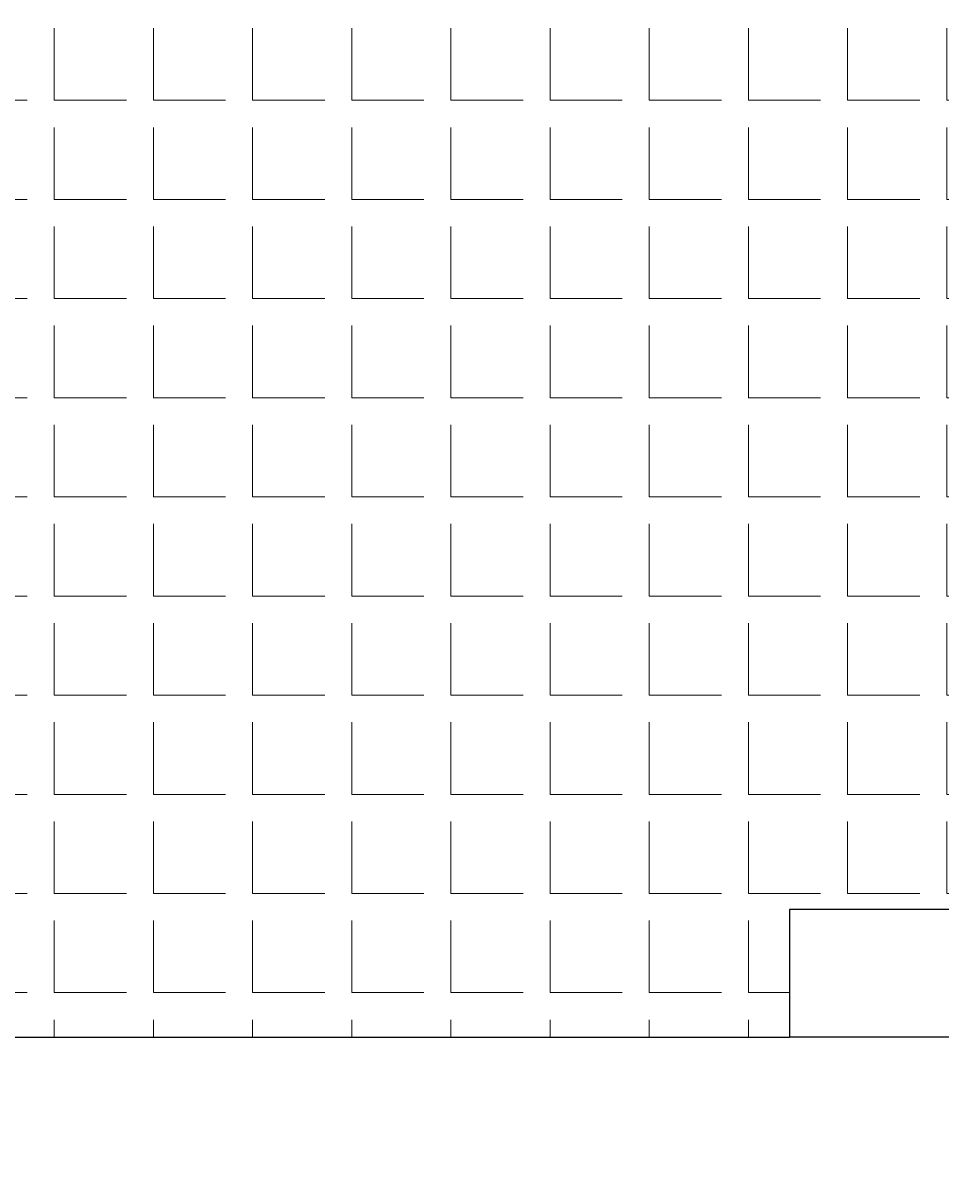
# Model space of a CAD drawing. Units: inches. Extents: x 84 to 1044, y -280 to 906.
# Tile 15 of 105: x 571 to 635, y -132 to -50. Entities that reach past the tile are written whole.
import ezdxf

# ---------------------------------------------------------------- set-up
doc = ezdxf.new("R2010")
doc.units = ezdxf.units.IN
doc.layers.add('A-ANNO-DIMS', color=2, linetype='Continuous', lineweight=18)
doc.layers.add('C-PROP', color=7, linetype='Continuous', lineweight=25)
doc.layers.add('L-HRDS-PATT', color=23, linetype='Continuous', lineweight=9, true_color=0xc2877b)
doc.styles.get("Standard").update_dxf_attribs({"font": 'arial.ttf'})
doc.dimstyles.get("Standard").update_dxf_attribs({"dimtxt": 0.18, "dimasz": 0.18, "dimexe": 0.18, "dimexo": 0.0625, "dimgap": 0.09, "dimtad": 0, "dimtih": 1, "dimtoh": 1, "dimdec": 4, "dimzin": 0, "dimdsep": 46, "dimtxsty": 'Standard', "dimcen": 0.09, "dimadec": 0, "dimazin": 0, "dimtfac": 1, "dimtdec": 4, "dimtofl": 0, "dimtmove": 0, "dimatfit": 3, "dimfxl": 1, "dimtolj": 1, "dimtzin": 0, "dimarcsym": 0})

# ---------------------------------------------------------------- blocks, each defined once
blk = doc.blocks.new('*D60')
at = {"layer": 'A-ANNO-DIMS', "color": 0, "lineweight": -2, "transparency": 16777216}
for p, q in [((134.179, -121.942), (134.179, -180.64)), ((992.074, -121.942), (992.074, -180.64)), ((134.359, -180.46), (562.733, -180.46)), ((991.894, -180.46), (563.521, -180.46))]:
    blk.add_line(p, q, dxfattribs=at)
at = {"layer": 'A-ANNO-DIMS', "color": 0, "transparency": 16777216}
for points in [[(134.359, -180.43), (134.359, -180.49), (134.179, -180.46)], [(991.894, -180.43), (991.894, -180.49), (992.074, -180.46)]]:
    blk.add_solid(points, dxfattribs=at)
at = {"layer": 'Defpoints', "color": 0, "transparency": 16777216}
for p in [(134.179, -121.88), (992.074, -121.88), (992.074, -180.46)]:
    blk.add_point(p, dxfattribs=at)
at = {"layer": 'A-ANNO-DIMS', "color": 0, "transparency": 16777216, "insert": (563.127, -180.46), "char_height": 0.18, "attachment_point": 5}
blk.add_mtext('\\A1;857.9', dxfattribs=at)

msp = doc.modelspace()

# ---------------------------------------------------------------- hatches: boundary and pattern name
at = {"layer": 'L-HRDS-PATT', "transparency": 33554567}
h = msp.add_hatch(dxfattribs=at)
h.set_pattern_fill('ANGLE', color=256)
h.set_pattern_definition([(0, (0, 0), (0, 6.985), [5.08, -1.905]), (90, (0, 0), (-6.985, 4e-16), [5.08, -1.905])])
h.paths.add_polyline_path([(650.074, 31.12), (504.574, 31.12), (504.574, -112.88), (504.574, -121.88), (624.574, -121.88), (624.574, -112.88), (650.074, -112.88)])

# ---------------------------------------------------------------- linework, layer by layer
at = {"layer": 'C-PROP'}
for p in [(624.574, -112.88), (504.574, -121.88)]:
    msp.add_line(p, (624.574, -121.88), dxfattribs=at)
for points in [[(143.179, -121.88), (134.179, -121.88), (134.179, 856.12), (992.074, 856.12), (992.074, -121.88), (624.574, -121.88)], [(143.179, -112.88), (143.179, 847.12), (983.074, 847.12), (983.074, -112.88), (624.574, -112.88)]]:
    msp.add_lwpolyline(points, dxfattribs=at)

# ---------------------------------------------------------------- dimensions: what is measured, and where the dimension line sits
at = {"layer": 'A-ANNO-DIMS'}
dim = msp.add_linear_dim(base=(992.074, -180.46), p1=(134.179, -121.88), p2=(992.074, -121.88), dimstyle='Standard', override={"dimdec": 1, "dimlfac": 1, "dimrnd": 0, "dimzin": 0, "dimdsep": 46, "dimlunit": 2}, dxfattribs=at)
dim.commit()
dim.dimension.update_dxf_attribs({"geometry": '*D60', "text_midpoint": (563.127, -180.46)})

doc.saveas('drawing.dxf')
